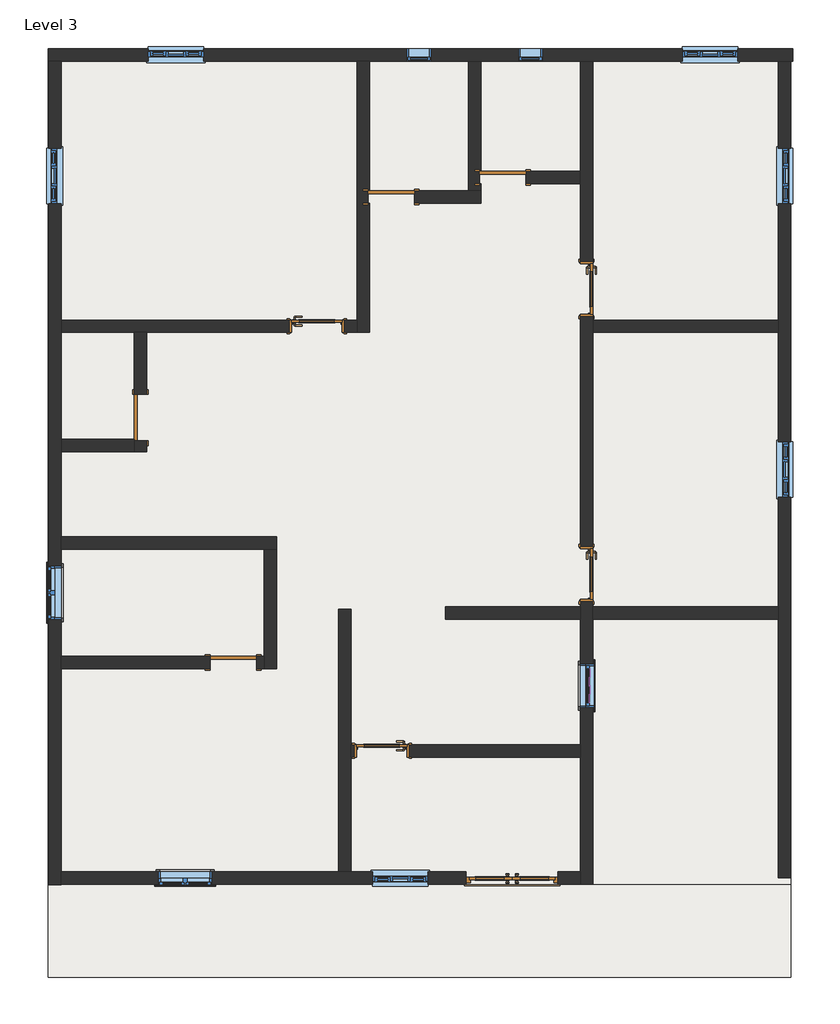
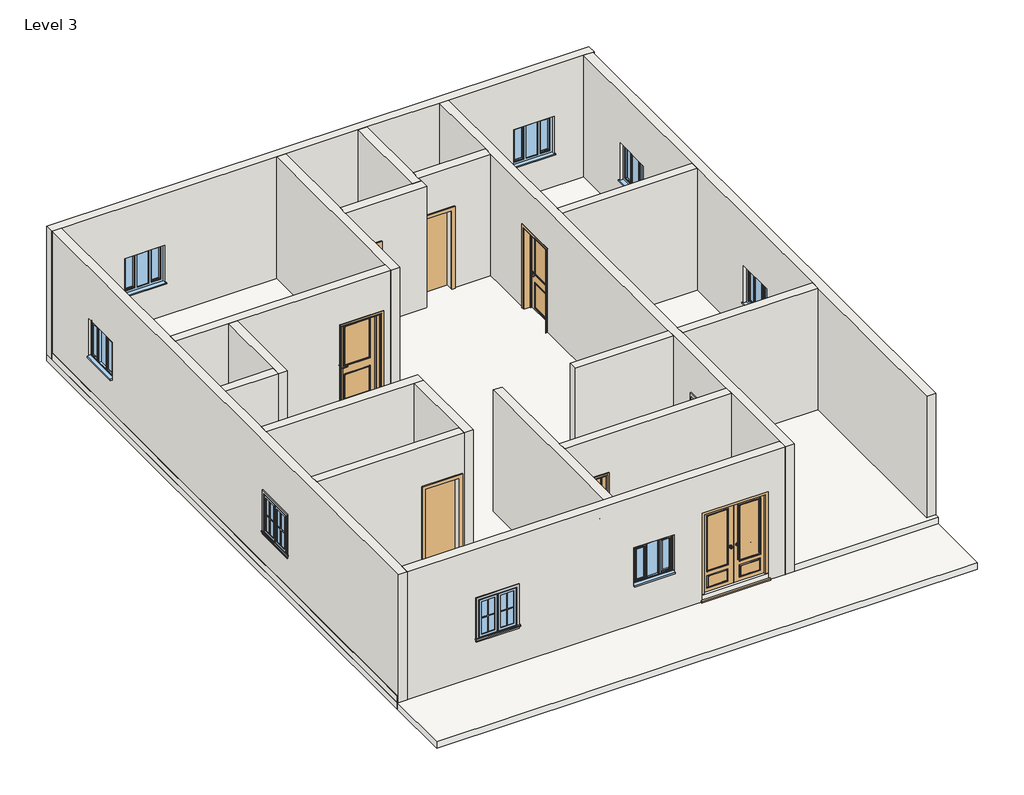
# One storey, incomplete: 19 walls, 12 proxies, 11 windows, 9 doors, 2 slabs, 1 roof.
"""IFC4 building model written with IfcOpenShell, lengths in millimetres."""

from ifc_helpers import new_model, si_unit, frame, origin, place, context, project, spatial, polyline, outline, extrude, faceted_brep, transform, mapped, element, save
from components import muntin_pattern_2x2_muntin_pattern_2x2_b3fe6957, muntin_pattern_2x2_muntin_pattern_2x2_3e0ecaf2, muntin_pattern_2x2_muntin_pattern_2x2_5f474966, trim_window_exterior_flat_with_sill_41619996, trim_window_exterior_flat_with_sill_68241f6a, trim_window_interior_flat_picture_frame_51c85655, trim_window_interior_flat_picture_frame_d3d93820, doors_extdbl_w_glazing_bars_2_1510x2110mm_e5cd3545, doors_extdbl_w_glazing_bars_2_1510x2110mm_b3535315, doors_intsgl_w_transome_910x2110mm_1071bad6, doors_intsgl_w_transome_910x2110mm_0d7ac49b, door_fadea3f2, door_53b1b562, window_085f26e1, window_c29befe5, window_4d695ea9, windows_tpl_plain_910x910mm_84e79c20

model = new_model("IFC4")

# Units and contexts
model_context = context("Model", 3, world=origin())
ifc_project = project(units=[si_unit("LENGTHUNIT", "METRE", prefix="MILLI")], contexts=[model_context])

# Site, building, storey
site = spatial("IfcSite", under=ifc_project)
building = spatial("IfcBuilding", under=site)
storey = spatial("IfcBuildingStorey", under=building, Name="Level 3", Elevation=6096.0)

# Proxies
placement = place(None, origin())
muntin_pattern_2x2_muntin_pattern_2x2_shape = muntin_pattern_2x2_muntin_pattern_2x2_b3fe6957(model_context)
element("IfcBuildingElementProxy", 1, Name="Muntin Pattern_2x2 : Muntin Pattern_2x2", ObjectType="Muntin Pattern_2x2 : Muntin Pattern_2x2", at=placement, inside=storey, context=model_context, shape_type="MappedRepresentation", body=[
    mapped(muntin_pattern_2x2_muntin_pattern_2x2_shape, transform((-4444.3565281, -6259.9254533, 7080.25), x_axis=(-1.0, 0.0, 0.0), y_axis=(0.0, -1.0, 0.0), z_axis=(0.0, 0.0, 1.0))),
])
element("IfcBuildingElementProxy", 2, Name="Muntin Pattern_2x2 : Muntin Pattern_2x2", ObjectType="Muntin Pattern_2x2 : Muntin Pattern_2x2", at=placement, inside=storey, context=model_context, shape_type="MappedRepresentation", body=[
    mapped(muntin_pattern_2x2_muntin_pattern_2x2_shape, transform((-6884.3440281, -1708.5629533, 7080.25), x_axis=(0.0, 1.0, 0.0), y_axis=(-1.0, 0.0, 0.0), z_axis=(0.0, 0.0, 1.0))),
])
muntin_pattern_2x2_muntin_pattern_2x2_2_shape = muntin_pattern_2x2_muntin_pattern_2x2_3e0ecaf2(model_context)
element("IfcBuildingElementProxy", 3, Name="Muntin Pattern_2x2 : Muntin Pattern_2x2", ObjectType="Muntin Pattern_2x2 : Muntin Pattern_2x2", at=placement, inside=storey, context=model_context, shape_type="MappedRepresentation", body=[
    mapped(muntin_pattern_2x2_muntin_pattern_2x2_2_shape, transform((-4872.9815281, -6259.9254533, 7080.25), x_axis=(1.0, 0.0, 0.0), y_axis=(0.0, 1.0, 0.0), z_axis=(0.0, 0.0, 1.0))),
])
element("IfcBuildingElementProxy", 4, Name="Muntin Pattern_2x2 : Muntin Pattern_2x2", ObjectType="Muntin Pattern_2x2 : Muntin Pattern_2x2", at=placement, inside=storey, context=model_context, shape_type="MappedRepresentation", body=[
    mapped(muntin_pattern_2x2_muntin_pattern_2x2_2_shape, transform((-6884.3440281, -1279.9379533, 7080.25), x_axis=(0.0, -1.0, 0.0), y_axis=(1.0, 0.0, 0.0), z_axis=(0.0, 0.0, 1.0))),
])
muntin_pattern_2x2_muntin_pattern_2x2_3_shape = muntin_pattern_2x2_muntin_pattern_2x2_5f474966(model_context)
element("IfcBuildingElementProxy", 5, Name="Muntin Pattern_2x2 : Muntin Pattern_2x2", ObjectType="Muntin Pattern_2x2 : Muntin Pattern_2x2", at=placement, inside=storey, context=model_context, shape_type="MappedRepresentation", body=[
    mapped(muntin_pattern_2x2_muntin_pattern_2x2_3_shape, transform((1989.809459, -3018.2504533, 7616.825), x_axis=(0.0, -1.0, 0.0), y_axis=(1.0, 0.0, 0.0), z_axis=(0.0, 0.0, 1.0))),
])
element("IfcBuildingElementProxy", 6, Name="Muntin Pattern_2x2 : Muntin Pattern_2x2", ObjectType="Muntin Pattern_2x2 : Muntin Pattern_2x2", at=placement, inside=storey, context=model_context, shape_type="MappedRepresentation", body=[
    mapped(muntin_pattern_2x2_muntin_pattern_2x2_3_shape, transform((1945.359459, -3018.2504533, 7086.6), x_axis=(0.0, -1.0, 0.0), y_axis=(1.0, 0.0, 0.0), z_axis=(0.0, 0.0, 1.0))),
])
trim_window_exterior_flat_with_sill_shape = trim_window_exterior_flat_with_sill_41619996(model_context)
element("IfcBuildingElementProxy", 7, Name="Trim-Window-Exterior-Flat : with Sill", ObjectType="Trim-Window-Exterior-Flat : with Sill", at=placement, inside=storey, context=model_context, shape_type="MappedRepresentation", body=[
    mapped(trim_window_exterior_flat_with_sill_shape, transform((-4658.6690281, -6269.4504533, 7924.8), x_axis=(1.0, 0.0, 0.0), y_axis=(0.0, 0.0, 1.0), z_axis=(0.0, -1.0, 0.0))),
])
element("IfcBuildingElementProxy", 8, Name="Trim-Window-Exterior-Flat : with Sill", ObjectType="Trim-Window-Exterior-Flat : with Sill", at=placement, inside=storey, context=model_context, shape_type="MappedRepresentation", body=[
    mapped(trim_window_exterior_flat_with_sill_shape, transform((-6893.8690281, -1494.2504533, 7924.8), x_axis=(0.0, -1.0, 0.0), y_axis=(0.0, 0.0, 1.0), z_axis=(-1.0, 0.0, 0.0))),
])
trim_window_exterior_flat_with_sill_2_shape = trim_window_exterior_flat_with_sill_68241f6a(model_context)
element("IfcBuildingElementProxy", 9, Name="Trim-Window-Exterior-Flat : with Sill", ObjectType="Trim-Window-Exterior-Flat : with Sill", at=placement, inside=storey, context=model_context, shape_type="MappedRepresentation", body=[
    mapped(trim_window_exterior_flat_with_sill_2_shape, transform((2024.734459, -3018.2504533, 8178.8), x_axis=(0.0, 1.0, 0.0), y_axis=(0.0, 0.0, 1.0), z_axis=(1.0, 0.0, 0.0))),
])
trim_window_interior_flat_picture_frame_shape = trim_window_interior_flat_picture_frame_51c85655(model_context)
element("IfcBuildingElementProxy", 10, Name="Trim-Window-Interior-Flat : Picture Frame", ObjectType="Trim-Window-Interior-Flat : Picture Frame", at=placement, inside=storey, context=model_context, shape_type="MappedRepresentation", body=[
    mapped(trim_window_interior_flat_picture_frame_shape, transform((-4658.6690281, -6066.2504533, 7924.8), x_axis=(-1.0, 0.0, 0.0), y_axis=(0.0, 0.0, 1.0), z_axis=(0.0, 1.0, 0.0))),
])
element("IfcBuildingElementProxy", 11, Name="Trim-Window-Interior-Flat : Picture Frame", ObjectType="Trim-Window-Interior-Flat : Picture Frame", at=placement, inside=storey, context=model_context, shape_type="MappedRepresentation", body=[
    mapped(trim_window_interior_flat_picture_frame_shape, transform((-6690.6690281, -1494.2504533, 7924.8), x_axis=(0.0, 1.0, 0.0), y_axis=(0.0, 0.0, 1.0), z_axis=(1.0, 0.0, 0.0))),
])
trim_window_interior_flat_picture_frame_2_shape = trim_window_interior_flat_picture_frame_d3d93820(model_context)
element("IfcBuildingElementProxy", 12, Name="Trim-Window-Interior-Flat : Picture Frame", ObjectType="Trim-Window-Interior-Flat : Picture Frame", at=placement, inside=storey, context=model_context, shape_type="MappedRepresentation", body=[
    mapped(trim_window_interior_flat_picture_frame_2_shape, transform((1821.534459, -3018.2504533, 8178.8), x_axis=(0.0, -1.0, 0.0), y_axis=(0.0, 0.0, 1.0), z_axis=(-1.0, 0.0, 0.0))),
])

# Doors
doors_extdbl_w_glazing_bars_2_1510x2110mm_shape = doors_extdbl_w_glazing_bars_2_1510x2110mm_e5cd3545(model_context)
doors_extdbl_w_glazing_bars_2_1510x2110mm_2_shape = doors_extdbl_w_glazing_bars_2_1510x2110mm_b3535315(model_context)
element("IfcDoor", 13, ObjectType="Doors_ExtDbl_w-Glazing_Bars_2 : 1510x2110mm", at=placement, inside=storey, context=model_context, shape_type="MappedRepresentation", body=[
    mapped(doors_extdbl_w_glazing_bars_2_1510x2110mm_shape, transform((703.934459, -6167.8504533, 6096.0), x_axis=(-1.0, 0.0, 0.0), y_axis=(0.0, -1.0, 0.0), z_axis=(0.0, 0.0, 1.0))),
    mapped(doors_extdbl_w_glazing_bars_2_1510x2110mm_2_shape, transform((703.934459, -6167.8504533, 6096.0), x_axis=(-1.0, 0.0, 0.0), y_axis=(0.0, -1.0, 0.0), z_axis=(0.0, 0.0, 1.0))),
])
doors_intsgl_w_transome_910x2110mm_shape = doors_intsgl_w_transome_910x2110mm_1071bad6(model_context)
element("IfcDoor", 14, ObjectType="Doors_IntSgl_w-Transome : 910x2110mm", at=placement, inside=storey, context=model_context, shape_type="MappedRepresentation", body=[
    mapped(doors_intsgl_w_transome_910x2110mm_shape, transform((-1432.8690281, -4085.0504533, 6096.0), x_axis=(-1.0, 0.0, 0.0), y_axis=(0.0, -1.0, 0.0), z_axis=(0.0, 0.0, 1.0))),
])
doors_intsgl_w_transome_910x2110mm_2_shape = doors_intsgl_w_transome_910x2110mm_0d7ac49b(model_context)
element("IfcDoor", 15, ObjectType="Doors_IntSgl_w-Transome : 910x2110mm", at=placement, inside=storey, context=model_context, shape_type="MappedRepresentation", body=[
    mapped(doors_intsgl_w_transome_910x2110mm_2_shape, transform((-2499.6690281, 2874.5495467, 6096.0), x_axis=(1.0, 0.0, 0.0), y_axis=(0.0, 1.0, 0.0), z_axis=(0.0, 0.0, 1.0))),
])
element("IfcDoor", 16, ObjectType="Doors_IntSgl_w-Transome : 910x2110mm", at=placement, inside=storey, context=model_context, shape_type="MappedRepresentation", body=[
    mapped(doors_intsgl_w_transome_910x2110mm_2_shape, transform((1923.134459, 3484.1495467, 6096.0), x_axis=(0.0, -1.0, 0.0), y_axis=(1.0, 0.0, 0.0), z_axis=(0.0, 0.0, 1.0))),
])
element("IfcDoor", 17, ObjectType="Doors_IntSgl_w-Transome : 910x2110mm", at=placement, inside=storey, context=model_context, shape_type="MappedRepresentation", body=[
    mapped(doors_intsgl_w_transome_910x2110mm_2_shape, transform((1923.134459, -1189.4504533, 6096.0), x_axis=(0.0, -1.0, 0.0), y_axis=(1.0, 0.0, 0.0), z_axis=(0.0, 0.0, 1.0))),
])
door_shape = door_fadea3f2(model_context)
element("IfcDoor", 18, ObjectType="Single-Flush : 30\" x 80\"", at=placement, inside=storey, context=model_context, shape_type="MappedRepresentation", body=[
    mapped(door_shape, transform((-3871.2690281, -2637.2504533, 6096.0), x_axis=(1.0, 0.0, 0.0), y_axis=(0.0, 1.0, 0.0), z_axis=(0.0, 0.0, 1.0))),
])
door_2_shape = door_53b1b562(model_context)
element("IfcDoor", 19, ObjectType="Single-Flush : 30\" x 80\"", at=placement, inside=storey, context=model_context, shape_type="MappedRepresentation", body=[
    mapped(door_2_shape, transform((-5395.2690281, 1375.9495467, 6096.0), x_axis=(0.0, -1.0, 0.0), y_axis=(1.0, 0.0, 0.0), z_axis=(0.0, 0.0, 1.0))),
])
element("IfcDoor", 20, ObjectType="Single-Flush : 30\" x 80\"", at=placement, inside=storey, context=model_context, shape_type="MappedRepresentation", body=[
    mapped(door_2_shape, transform((-1280.4690281, 4995.4495467, 6096.0), x_axis=(-1.0, 0.0, 0.0), y_axis=(0.0, -1.0, 0.0), z_axis=(0.0, 0.0, 1.0))),
])
element("IfcDoor", 21, ObjectType="Single-Flush : 30\" x 80\"", at=placement, inside=storey, context=model_context, shape_type="MappedRepresentation", body=[
    mapped(door_2_shape, transform((548.3309719, 5312.9495467, 6096.0), x_axis=(-1.0, 0.0, 0.0), y_axis=(0.0, -1.0, 0.0), z_axis=(0.0, 0.0, 1.0))),
])

# Roof
element("IfcRoof", 22, ObjectType="Generic - 12\"", at=placement, inside=storey, context=model_context, shape_type="SweptSolid", body=[
    extrude(outline(polyline([(-6906.5690281, 7421.1495467), (5272.7309719, 7421.1495467), (5272.7309719, -6269.4504533), (-6906.5690281, -6269.4504533), (-6906.5690281, 7421.1495467)])), frame((0.0, 0.0, 6096.0), z_axis=(0.0, 0.0, 1.0), x_axis=(1.0, 0.0, 0.0)), (0.0, 0.0, 1.0), 152.4),
])

# Slabs
element("IfcSlab", 23, ObjectType="Generic - 12\"", at=placement, inside=storey, context=model_context, shape_type="SweptSolid", body=[
    extrude(outline(polyline([(5272.7309719, 7421.1495467), (5272.7309719, -6269.4504533), (-6906.5690281, -6269.4504533), (-6906.5690281, 7421.1495467), (5272.7309719, 7421.1495467)])), frame((0.0, 0.0, 5943.6), z_axis=(0.0, 0.0, 1.0), x_axis=(1.0, 0.0, 0.0)), (0.0, 0.0, 1.0), 152.4),
])
element("IfcSlab", 24, ObjectType="Generic - 12\"", at=placement, inside=storey, context=model_context, shape_type="SweptSolid", body=[
    extrude(outline(polyline([(5272.7309719, -6269.4504533), (5272.7309719, -7799.0240652), (-6906.5690281, -7799.0240652), (-6906.5690281, -6269.4504533), (5272.7309719, -6269.4504533)])), frame((0.0, 0.0, 5943.6), z_axis=(0.0, 0.0, 1.0), x_axis=(1.0, 0.0, 0.0)), (0.0, 0.0, 1.0), 152.4),
])

# Walls
element("IfcWall", 25, ObjectType="4.5\" p", at=placement, inside=storey, context=model_context, shape_type="Brep", body=[
    faceted_brep([(-1839.2690281, 7217.9495467, 6096.0), (-1839.2690281, 2976.1495467, 6096.0), (-1839.2690281, 2772.9495467, 6096.0), (-1839.2690281, 2772.9495467, 9144.0), (-1839.2690281, 2976.1495467, 9144.0), (-1839.2690281, 7217.9495467, 9144.0), (-1636.0690281, 7217.9495467, 9144.0), (-1636.0690281, 5097.0495467, 9144.0), (-1636.0690281, 4893.8495467, 9144.0), (-1636.0690281, 2772.9495467, 9144.0), (-1636.0690281, 2772.9495467, 6096.0), (-1636.0690281, 4893.8495467, 6096.0), (-1636.0690281, 4893.8495467, 8128.0), (-1636.0690281, 5097.0495467, 8128.0), (-1636.0690281, 5097.0495467, 6096.0), (-1636.0690281, 7217.9495467, 6096.0), (-1661.4690281, 5097.0495467, 6096.0), (-1661.4690281, 4893.8495467, 6096.0), (-1661.4690281, 5097.0495467, 8128.0), (-1661.4690281, 4893.8495467, 8128.0)], [[[0, 1, 2, 3, 4, 5]], [[6, 7, 8, 9, 10, 11, 12, 13, 14, 15]], [[2, 1, 0, 15, 14, 16, 17, 11, 10]], [[5, 4, 3, 9, 8, 7, 6]], [[0, 5, 6, 15]], [[3, 2, 10, 9]], [[18, 16, 14, 13]], [[17, 19, 12, 11]], [[19, 18, 13, 12]], [[16, 18, 19, 17]]]),
])
element("IfcWall", 26, ObjectType="4.5\" p", at=placement, inside=storey, context=model_context, shape_type="Brep", body=[
    faceted_brep([(-1839.2690281, 2772.9495467, 9144.0), (-5293.6690281, 2772.9495467, 9144.0), (-5496.8690281, 2772.9495467, 9144.0), (-6690.6690281, 2772.9495467, 9144.0), (-6690.6690281, 2772.9495467, 6096.0), (-5496.8690281, 2772.9495467, 6096.0), (-5293.6690281, 2772.9495467, 6096.0), (-2954.6690281, 2772.9495467, 6096.0), (-2954.6690281, 2772.9495467, 8206.0), (-2044.6690281, 2772.9495467, 8206.0), (-2044.6690281, 2772.9495467, 6096.0), (-1839.2690281, 2772.9495467, 6096.0), (-6690.6690281, 2976.1495467, 9144.0), (-1839.2690281, 2976.1495467, 9144.0), (-1839.2690281, 2976.1495467, 6096.0), (-2044.6690281, 2976.1495467, 6096.0), (-2044.6690281, 2976.1495467, 8206.0), (-2954.6690281, 2976.1495467, 8206.0), (-2954.6690281, 2976.1495467, 6096.0), (-6690.6690281, 2976.1495467, 6096.0)], [[[0, 1, 2, 3, 4, 5, 6, 7, 8, 9, 10, 11]], [[12, 13, 14, 15, 16, 17, 18, 19]], [[4, 19, 18, 7, 6, 5]], [[14, 11, 10, 15]], [[3, 2, 1, 0, 13, 12]], [[0, 11, 14, 13]], [[4, 3, 12, 19]], [[9, 16, 15, 10]], [[16, 9, 8, 17]], [[17, 8, 7, 18]]]),
])
element("IfcWall", 27, ObjectType="4.5\" p", at=placement, inside=storey, context=model_context, shape_type="Brep", body=[
    faceted_brep([(-5496.8690281, 994.9495467, 8128.0), (-5496.8690281, 994.9495467, 6096.0), (-5496.8690281, 817.1495467, 6096.0), (-5496.8690281, 817.1495467, 9144.0), (-5496.8690281, 1020.3495467, 9144.0), (-5496.8690281, 2772.9495467, 9144.0), (-5496.8690281, 2772.9495467, 6096.0), (-5496.8690281, 1756.9495467, 6096.0), (-5496.8690281, 1756.9495467, 8128.0), (-5293.6690281, 817.1495467, 6096.0), (-5293.6690281, 994.9495467, 6096.0), (-5293.6690281, 994.9495467, 8128.0), (-5293.6690281, 1756.9495467, 8128.0), (-5293.6690281, 1756.9495467, 6096.0), (-5293.6690281, 2772.9495467, 6096.0), (-5293.6690281, 2772.9495467, 9144.0), (-5293.6690281, 817.1495467, 9144.0)], [[[0, 1, 2, 3, 4, 5, 6, 7, 8]], [[9, 10, 11, 12, 13, 14, 15, 16]], [[7, 6, 14, 13]], [[2, 1, 10, 9]], [[5, 4, 3, 16, 15]], [[6, 5, 15, 14]], [[3, 2, 9, 16]], [[11, 10, 1, 0]], [[12, 11, 0, 8]], [[13, 12, 8, 7]]]),
])
element("IfcWall", 28, ObjectType="4.5\" p", at=placement, inside=storey, context=model_context, shape_type="SweptSolid", body=[
    extrude(outline(polyline([(-5496.8690281, 817.1495467), (-6690.6690281, 817.1495467), (-6690.6690281, 1020.3495467), (-5496.8690281, 1020.3495467), (-5496.8690281, 817.1495467)])), frame((0.0, 0.0, 6096.0), z_axis=(0.0, 0.0, 1.0), x_axis=(1.0, 0.0, 0.0)), (0.0, 0.0, 1.0), 3048.0),
])
element("IfcWall", 29, ObjectType="4.5\" p", at=placement, inside=storey, context=model_context, shape_type="Brep", body=[
    faceted_brep([(-6690.6690281, -783.0504533, 6096.0), (-3363.2690281, -783.0504533, 6096.0), (-3160.0690281, -783.0504533, 6096.0), (-3160.0690281, -783.0504533, 9144.0), (-3363.2690281, -783.0504533, 9144.0), (-6690.6690281, -783.0504533, 9144.0), (-6690.6690281, -579.8504533, 6096.0), (-6690.6690281, -579.8504533, 9144.0), (-3160.0690281, -579.8504533, 9144.0), (-3160.0690281, -579.8504533, 6096.0)], [[[0, 1, 2, 3, 4, 5]], [[6, 7, 8, 9]], [[2, 1, 0, 6, 9]], [[5, 4, 3, 8, 7]], [[0, 5, 7, 6]], [[3, 2, 9, 8]]]),
])
element("IfcWall", 30, ObjectType="4.5\" p", at=placement, inside=storey, context=model_context, shape_type="Brep", body=[
    faceted_brep([(-3363.2690281, -783.0504533, 6096.0), (-3363.2690281, -2535.6504533, 6096.0), (-3363.2690281, -2738.8504533, 6096.0), (-3363.2690281, -2738.8504533, 9144.0), (-3363.2690281, -2535.6504533, 9144.0), (-3363.2690281, -783.0504533, 9144.0), (-3160.0690281, -783.0504533, 6096.0), (-3160.0690281, -783.0504533, 9144.0), (-3160.0690281, -2738.8504533, 9144.0), (-3160.0690281, -2738.8504533, 6096.0)], [[[0, 1, 2, 3, 4, 5]], [[6, 7, 8, 9]], [[2, 1, 0, 6, 9]], [[5, 4, 3, 8, 7]], [[0, 5, 7, 6]], [[3, 2, 9, 8]]]),
])
element("IfcWall", 31, ObjectType="4.5\" p", at=placement, inside=storey, context=model_context, shape_type="SweptSolid", body=[
    extrude(outline(polyline([(8128.0, -3490.2690281), (6096.0, -3490.2690281), (6096.0, -3363.2690281), (9144.0, -3363.2690281), (9144.0, -6690.6690281), (6096.0, -6690.6690281), (6096.0, -4252.2690281), (8128.0, -4252.2690281), (8128.0, -3490.2690281)])), frame((0.0, -2738.8504533, 0.0), z_axis=(0.0, 1.0, 0.0), x_axis=(0.0, 0.0, 1.0)), (0.0, 0.0, 1.0), 203.2),
])
element("IfcWall", 32, ObjectType="4.5\" p", at=placement, inside=storey, context=model_context, shape_type="Brep", body=[
    faceted_brep([(192.7309719, 4893.8495467, 9144.0), (-1636.0690281, 4893.8495467, 9144.0), (-1636.0690281, 4893.8495467, 8128.0), (-899.4690281, 4893.8495467, 8128.0), (-899.4690281, 4893.8495467, 6096.0), (192.7309719, 4893.8495467, 6096.0), (-1636.0690281, 5097.0495467, 9144.0), (-10.4690281, 5097.0495467, 9144.0), (192.7309719, 5097.0495467, 9144.0), (192.7309719, 5097.0495467, 6096.0), (-10.4690281, 5097.0495467, 6096.0), (-899.4690281, 5097.0495467, 6096.0), (-899.4690281, 5097.0495467, 8128.0), (-1636.0690281, 5097.0495467, 8128.0)], [[[0, 1, 2, 3, 4, 5]], [[6, 7, 8, 9, 10, 11, 12, 13]], [[9, 5, 4, 11, 10]], [[1, 0, 8, 7, 6]], [[1, 6, 13, 2]], [[0, 5, 9, 8]], [[12, 3, 2, 13]], [[3, 12, 11, 4]]]),
])
element("IfcWall", 33, ObjectType="4.5\" p", at=placement, inside=storey, context=model_context, shape_type="Brep", body=[
    faceted_brep([(-10.4690281, 7217.9495467, 6096.0), (-10.4690281, 5097.0495467, 6096.0), (-10.4690281, 5097.0495467, 9144.0), (-10.4690281, 7217.9495467, 9144.0), (192.7309719, 7217.9495467, 9144.0), (192.7309719, 5414.5495467, 9144.0), (192.7309719, 5211.3495467, 9144.0), (192.7309719, 5097.0495467, 9144.0), (192.7309719, 5097.0495467, 6096.0), (192.7309719, 5211.3495467, 6096.0), (192.7309719, 5211.3495467, 8128.0), (192.7309719, 5414.5495467, 8128.0), (192.7309719, 5414.5495467, 6096.0), (192.7309719, 7217.9495467, 6096.0), (167.3309719, 5414.5495467, 6096.0), (167.3309719, 5211.3495467, 6096.0), (167.3309719, 5414.5495467, 8128.0), (167.3309719, 5211.3495467, 8128.0)], [[[0, 1, 2, 3]], [[4, 5, 6, 7, 8, 9, 10, 11, 12, 13]], [[1, 0, 13, 12, 14, 15, 9, 8]], [[3, 2, 7, 6, 5, 4]], [[2, 1, 8, 7]], [[0, 3, 4, 13]], [[16, 14, 12, 11]], [[15, 17, 10, 9]], [[17, 16, 11, 10]], [[14, 16, 17, 15]]]),
])
element("IfcWall", 34, ObjectType="4.5\" p", at=placement, inside=storey, context=model_context, shape_type="Brep", body=[
    faceted_brep([(1821.534459, -6269.4504533, 9144.0), (1821.534459, -6066.2504533, 9144.0), (1821.534459, -4186.6504533, 9144.0), (1821.534459, -3983.4504533, 9144.0), (1821.534459, -1926.0504533, 9144.0), (1821.534459, -1722.8504533, 9144.0), (1821.534459, 5211.3495467, 9144.0), (1821.534459, 5414.5495467, 9144.0), (1821.534459, 7217.9495467, 9144.0), (1821.534459, 7217.9495467, 6096.0), (1821.534459, 5414.5495467, 6096.0), (1821.534459, 5211.3495467, 6096.0), (1821.534459, 3939.1495467, 6096.0), (1821.534459, 3939.1495467, 8206.0), (1821.534459, 3029.1495467, 8206.0), (1821.534459, 3029.1495467, 6096.0), (1821.534459, -734.4504533, 6096.0), (1821.534459, -734.4504533, 8206.0), (1821.534459, -1644.4504533, 8206.0), (1821.534459, -1644.4504533, 6096.0), (1821.534459, -1722.8504533, 6096.0), (1821.534459, -1926.0504533, 6096.0), (1821.534459, -3983.4504533, 6096.0), (1821.534459, -4186.6504533, 6096.0), (1821.534459, -6066.2504533, 6096.0), (1821.534459, -6269.4504533, 6096.0), (1821.534459, -2662.6504533, 8178.8), (1821.534459, -3373.8504533, 8178.8), (1821.534459, -3373.8504533, 7010.4), (1821.534459, -2662.6504533, 7010.4), (2024.734459, 7217.9495467, 9144.0), (2024.734459, 2976.1495467, 9144.0), (2024.734459, 2772.9495467, 9144.0), (2024.734459, -1722.8504533, 9144.0), (2024.734459, -1926.0504533, 9144.0), (2024.734459, -6269.4504533, 9144.0), (2024.734459, -6269.4504533, 6096.0), (2024.734459, -1926.0504533, 6096.0), (2024.734459, -1722.8504533, 6096.0), (2024.734459, -1644.4504533, 6096.0), (2024.734459, -1644.4504533, 8206.0), (2024.734459, -734.4504533, 8206.0), (2024.734459, -734.4504533, 6096.0), (2024.734459, 2772.9495467, 6096.0), (2024.734459, 2976.1495467, 6096.0), (2024.734459, 3029.1495467, 6096.0), (2024.734459, 3029.1495467, 8206.0), (2024.734459, 3939.1495467, 8206.0), (2024.734459, 3939.1495467, 6096.0), (2024.734459, 7217.9495467, 6096.0), (2024.734459, -2662.6504533, 8178.8), (2024.734459, -2662.6504533, 7010.4), (2024.734459, -3373.8504533, 7010.4), (2024.734459, -3373.8504533, 8178.8)], [[[0, 1, 2, 3, 4, 5, 6, 7, 8, 9, 10, 11, 12, 13, 14, 15, 16, 17, 18, 19, 20, 21, 22, 23, 24, 25], [26, 27, 28, 29]], [[30, 31, 32, 33, 34, 35, 36, 37, 38, 39, 40, 41, 42, 43, 44, 45, 46, 47, 48, 49], [50, 51, 52, 53]], [[9, 49, 48, 12, 11, 10]], [[15, 45, 44, 43, 42, 16]], [[36, 25, 24, 23, 22, 21, 20, 19, 39, 38, 37]], [[8, 7, 6, 5, 4, 3, 2, 1, 0, 35, 34, 33, 32, 31, 30]], [[9, 8, 30, 49]], [[14, 46, 45, 15]], [[46, 14, 13, 47]], [[47, 13, 12, 48]], [[18, 40, 39, 19]], [[40, 18, 17, 41]], [[41, 17, 16, 42]], [[0, 25, 36, 35]], [[51, 50, 26, 29]], [[52, 51, 29, 28]], [[53, 52, 28, 27]], [[50, 53, 27, 26]]]),
])
element("IfcWall", 35, ObjectType="4.5\" p", at=placement, inside=storey, context=model_context, shape_type="SweptSolid", body=[
    extrude(outline(polyline([(-391.4690281, -1926.0504533), (-391.4690281, -1722.8504533), (1821.534459, -1722.8504533), (1821.534459, -1926.0504533), (-391.4690281, -1926.0504533)])), frame((0.0, 0.0, 6096.0), z_axis=(0.0, 0.0, 1.0), x_axis=(1.0, 0.0, 0.0)), (0.0, 0.0, 1.0), 3048.0),
    extrude(outline(polyline([(5069.5309719, -1722.8504533), (5069.5309719, -1926.0504533), (2024.734459, -1926.0504533), (2024.734459, -1722.8504533), (5069.5309719, -1722.8504533)])), frame((0.0, 0.0, 6096.0), z_axis=(0.0, 0.0, 1.0), x_axis=(1.0, 0.0, 0.0)), (0.0, 0.0, 1.0), 3048.0),
])
element("IfcWall", 36, ObjectType="4.5\" p", at=placement, inside=storey, context=model_context, shape_type="SweptSolid", body=[
    extrude(outline(polyline([(5069.5309719, 2772.9495467), (2024.734459, 2772.9495467), (2024.734459, 2976.1495467), (5069.5309719, 2976.1495467), (5069.5309719, 2772.9495467)])), frame((0.0, 0.0, 6096.0), z_axis=(0.0, 0.0, 1.0), x_axis=(1.0, 0.0, 0.0)), (0.0, 0.0, 1.0), 3048.0),
])
element("IfcWall", 37, ObjectType="4.5\" p", at=placement, inside=storey, context=model_context, shape_type="SweptSolid", body=[
    extrude(outline(polyline([(9144.0, 1821.534459), (9144.0, 192.7309719), (8128.0, 192.7309719), (8128.0, 929.3309719), (6096.0, 929.3309719), (6096.0, 1821.534459), (9144.0, 1821.534459)])), frame((0.0, 5211.3495467, 0.0), z_axis=(0.0, 1.0, 0.0), x_axis=(0.0, 0.0, 1.0)), (0.0, 0.0, 1.0), 203.2),
])
element("IfcWall", 38, ObjectType="4.5\" p", at=placement, inside=storey, context=model_context, shape_type="Brep", body=[
    faceted_brep([(-1940.8690281, -6066.2504533, 6096.0), (-1940.8690281, -4186.6504533, 6096.0), (-1940.8690281, -3983.4504533, 6096.0), (-1940.8690281, -1760.9504533, 6096.0), (-1940.8690281, -1760.9504533, 9144.0), (-1940.8690281, -3983.4504533, 9144.0), (-1940.8690281, -4186.6504533, 9144.0), (-1940.8690281, -6066.2504533, 9144.0), (-2144.0690281, -6066.2504533, 6096.0), (-2144.0690281, -6066.2504533, 9144.0), (-2144.0690281, -1760.9504533, 9144.0), (-2144.0690281, -1760.9504533, 6096.0)], [[[0, 1, 2, 3, 4, 5, 6, 7]], [[8, 9, 10, 11]], [[3, 2, 1, 0, 8, 11]], [[4, 3, 11, 10]], [[7, 6, 5, 4, 10, 9]], [[0, 7, 9, 8]]]),
])
element("IfcWall", 39, ObjectType="4.5\" p", at=placement, inside=storey, context=model_context, shape_type="SweptSolid", body=[
    extrude(outline(polyline([(9144.0, 1821.534459), (9144.0, -1940.8690281), (6096.0, -1940.8690281), (6096.0, -1887.8690281), (8206.0, -1887.8690281), (8206.0, -977.8690281), (6096.0, -977.8690281), (6096.0, 1821.534459), (9144.0, 1821.534459)])), frame((0.0, -4186.6504533, 0.0), z_axis=(0.0, 1.0, 0.0), x_axis=(0.0, 0.0, 1.0)), (0.0, 0.0, 1.0), 203.2),
])
element("IfcWall", 40, ObjectType="9\"", at=placement, inside=storey, context=model_context, shape_type="Brep", body=[
    faceted_brep([(5069.5309719, 7217.9495467, 6096.0), (5069.5309719, 2976.1495467, 6096.0), (5069.5309719, 2772.9495467, 6096.0), (5069.5309719, -1722.8504533, 6096.0), (5069.5309719, -1926.0504533, 6096.0), (5069.5309719, -6167.8504533, 6096.0), (5069.5309719, -6167.8504533, 9144.0), (5069.5309719, -1926.0504533, 9144.0), (5069.5309719, -1722.8504533, 9144.0), (5069.5309719, 2772.9495467, 9144.0), (5069.5309719, 2976.1495467, 9144.0), (5069.5309719, 7217.9495467, 9144.0), (5069.5309719, 980.0495467, 7920.4), (5069.5309719, 70.0495467, 7920.4), (5069.5309719, 70.0495467, 7010.4), (5069.5309719, 980.0495467, 7010.4), (5069.5309719, 5793.3495467, 7920.4), (5069.5309719, 4883.3495467, 7920.4), (5069.5309719, 4883.3495467, 7010.4), (5069.5309719, 5793.3495467, 7010.4), (5272.7309719, 7217.9495467, 6096.0), (5272.7309719, 7217.9495467, 9144.0), (5272.7309719, -6167.8504533, 9144.0), (5272.7309719, -6167.8504533, 6096.0), (5272.7309719, 980.0495467, 7920.4), (5272.7309719, 980.0495467, 7010.4), (5272.7309719, 70.0495467, 7010.4), (5272.7309719, 70.0495467, 7920.4), (5272.7309719, 5793.3495467, 7920.4), (5272.7309719, 5793.3495467, 7010.4), (5272.7309719, 4883.3495467, 7010.4), (5272.7309719, 4883.3495467, 7920.4)], [[[0, 1, 2, 3, 4, 5, 6, 7, 8, 9, 10, 11], [12, 13, 14, 15], [16, 17, 18, 19]], [[20, 21, 22, 23], [24, 25, 26, 27], [28, 29, 30, 31]], [[5, 4, 3, 2, 1, 0, 20, 23]], [[6, 5, 23, 22]], [[11, 10, 9, 8, 7, 6, 22, 21]], [[0, 11, 21, 20]], [[25, 24, 12, 15]], [[26, 25, 15, 14]], [[27, 26, 14, 13]], [[24, 27, 13, 12]], [[29, 28, 16, 19]], [[30, 29, 19, 18]], [[31, 30, 18, 17]], [[28, 31, 17, 16]]]),
])
element("IfcWall", 41, ObjectType="9\" wall", at=placement, inside=storey, context=model_context, shape_type="Brep", body=[
    faceted_brep([(-6906.5690281, 7217.9495467, 6096.0), (-6893.8690281, 7217.9495467, 6096.0), (-6690.6690281, 7217.9495467, 6096.0), (-1839.2690281, 7217.9495467, 6096.0), (-1636.0690281, 7217.9495467, 6096.0), (-10.4690281, 7217.9495467, 6096.0), (192.7309719, 7217.9495467, 6096.0), (1821.534459, 7217.9495467, 6096.0), (2024.734459, 7217.9495467, 6096.0), (5069.5309719, 7217.9495467, 6096.0), (5272.7309719, 7217.9495467, 6096.0), (5310.8309719, 7217.9495467, 6096.0), (5310.8309719, 7217.9495467, 9144.0), (5272.7309719, 7217.9495467, 9144.0), (5069.5309719, 7217.9495467, 9144.0), (2024.734459, 7217.9495467, 9144.0), (1821.534459, 7217.9495467, 9144.0), (192.7309719, 7217.9495467, 9144.0), (-10.4690281, 7217.9495467, 9144.0), (-1636.0690281, 7217.9495467, 9144.0), (-1839.2690281, 7217.9495467, 9144.0), (-6690.6690281, 7217.9495467, 9144.0), (-6893.8690281, 7217.9495467, 9144.0), (-6906.5690281, 7217.9495467, 9144.0), (-5266.0690281, 7217.9495467, 7920.4), (-4356.0690281, 7217.9495467, 7920.4), (-4356.0690281, 7217.9495467, 7010.4), (-5266.0690281, 7217.9495467, 7010.4), (3496.9309719, 7217.9495467, 7920.4), (4406.9309719, 7217.9495467, 7920.4), (4406.9309719, 7217.9495467, 7010.4), (3496.9309719, 7217.9495467, 7010.4), (-1026.4690281, 7217.9495467, 7620.0), (-620.0690281, 7217.9495467, 7620.0), (-620.0690281, 7217.9495467, 7010.4), (-1026.4690281, 7217.9495467, 7010.4), (803.9327155, 7217.9495467, 7620.0), (1210.3327155, 7217.9495467, 7620.0), (1210.3327155, 7217.9495467, 7010.4), (803.9327155, 7217.9495467, 7010.4), (-6906.5690281, 7421.1495467, 6096.0), (-6906.5690281, 7421.1495467, 9144.0), (5310.8309719, 7421.1495467, 9144.0), (5310.8309719, 7421.1495467, 6096.0), (-5266.0690281, 7421.1495467, 7920.4), (-5266.0690281, 7421.1495467, 7010.4), (-4356.0690281, 7421.1495467, 7010.4), (-4356.0690281, 7421.1495467, 7920.4), (3496.9309719, 7421.1495467, 7920.4), (3496.9309719, 7421.1495467, 7010.4), (4406.9309719, 7421.1495467, 7010.4), (4406.9309719, 7421.1495467, 7920.4), (-1026.4690281, 7421.1495467, 7620.0), (-1026.4690281, 7421.1495467, 7010.4), (-620.0690281, 7421.1495467, 7010.4), (-620.0690281, 7421.1495467, 7620.0), (803.9327155, 7421.1495467, 7620.0), (803.9327155, 7421.1495467, 7010.4), (1210.3327155, 7421.1495467, 7010.4), (1210.3327155, 7421.1495467, 7620.0)], [[[0, 1, 2, 3, 4, 5, 6, 7, 8, 9, 10, 11, 12, 13, 14, 15, 16, 17, 18, 19, 20, 21, 22, 23], [24, 25, 26, 27], [28, 29, 30, 31], [32, 33, 34, 35], [36, 37, 38, 39]], [[40, 41, 42, 43], [44, 45, 46, 47], [48, 49, 50, 51], [52, 53, 54, 55], [56, 57, 58, 59]], [[11, 10, 9, 8, 7, 6, 5, 4, 3, 2, 1, 0, 40, 43]], [[12, 11, 43, 42]], [[23, 22, 21, 20, 19, 18, 17, 16, 15, 14, 13, 12, 42, 41]], [[0, 23, 41, 40]], [[45, 44, 24, 27]], [[46, 45, 27, 26]], [[47, 46, 26, 25]], [[44, 47, 25, 24]], [[49, 48, 28, 31]], [[50, 49, 31, 30]], [[51, 50, 30, 29]], [[48, 51, 29, 28]], [[53, 52, 32, 35]], [[54, 53, 35, 34]], [[55, 54, 34, 33]], [[52, 55, 33, 32]], [[57, 56, 36, 39]], [[58, 57, 39, 38]], [[59, 58, 38, 37]], [[56, 59, 37, 36]]]),
])
element("IfcWall", 42, ObjectType="9\" wall", at=placement, inside=storey, context=model_context, shape_type="Brep", body=[
    faceted_brep([(-6893.8690281, 7217.9495467, 6096.0), (-6893.8690281, -6282.1504533, 6096.0), (-6893.8690281, -6282.1504533, 9144.0), (-6893.8690281, 7217.9495467, 9144.0), (-6893.8690281, -1062.4504533, 7924.8), (-6893.8690281, -1926.0504533, 7924.8), (-6893.8690281, -1926.0504533, 7010.4), (-6893.8690281, -1062.4504533, 7010.4), (-6893.8690281, 4883.3495467, 7920.4), (-6893.8690281, 4883.3495467, 7010.4), (-6893.8690281, 5793.3495467, 7010.4), (-6893.8690281, 5793.3495467, 7920.4), (-6690.6690281, 7217.9495467, 6096.0), (-6690.6690281, 7217.9495467, 9144.0), (-6690.6690281, 2976.1495467, 9144.0), (-6690.6690281, 2772.9495467, 9144.0), (-6690.6690281, 1020.3495467, 9144.0), (-6690.6690281, 817.1495467, 9144.0), (-6690.6690281, -579.8504533, 9144.0), (-6690.6690281, -783.0504533, 9144.0), (-6690.6690281, -2535.6504533, 9144.0), (-6690.6690281, -2738.8504533, 9144.0), (-6690.6690281, -6066.2504533, 9144.0), (-6690.6690281, -6269.4504533, 9144.0), (-6690.6690281, -6282.1504533, 9144.0), (-6690.6690281, -6282.1504533, 6096.0), (-6690.6690281, -6269.4504533, 6096.0), (-6690.6690281, -6066.2504533, 6096.0), (-6690.6690281, -2738.8504533, 6096.0), (-6690.6690281, -2535.6504533, 6096.0), (-6690.6690281, -783.0504533, 6096.0), (-6690.6690281, -579.8504533, 6096.0), (-6690.6690281, 817.1495467, 6096.0), (-6690.6690281, 1020.3495467, 6096.0), (-6690.6690281, 2772.9495467, 6096.0), (-6690.6690281, 2976.1495467, 6096.0), (-6690.6690281, -1062.4504533, 7924.8), (-6690.6690281, -1062.4504533, 7010.4), (-6690.6690281, -1926.0504533, 7010.4), (-6690.6690281, -1926.0504533, 7924.8), (-6690.6690281, 4883.3495467, 7920.4), (-6690.6690281, 5793.3495467, 7920.4), (-6690.6690281, 5793.3495467, 7010.4), (-6690.6690281, 4883.3495467, 7010.4)], [[[0, 1, 2, 3], [4, 5, 6, 7], [8, 9, 10, 11]], [[12, 13, 14, 15, 16, 17, 18, 19, 20, 21, 22, 23, 24, 25, 26, 27, 28, 29, 30, 31, 32, 33, 34, 35], [36, 37, 38, 39], [40, 41, 42, 43]], [[1, 0, 12, 35, 34, 33, 32, 31, 30, 29, 28, 27, 26, 25]], [[2, 1, 25, 24]], [[3, 2, 24, 23, 22, 21, 20, 19, 18, 17, 16, 15, 14, 13]], [[0, 3, 13, 12]], [[37, 36, 4, 7]], [[38, 37, 7, 6]], [[39, 38, 6, 5]], [[36, 39, 5, 4]], [[9, 8, 40, 43]], [[10, 9, 43, 42]], [[11, 10, 42, 41]], [[8, 11, 41, 40]]]),
])
element("IfcWall", 43, ObjectType="9\" wall", at=placement, inside=storey, context=model_context, shape_type="Brep", body=[
    faceted_brep([(1821.534459, -6269.4504533, 9144.0), (-6690.6690281, -6269.4504533, 9144.0), (-6690.6690281, -6269.4504533, 6096.0), (-51.065541, -6269.4504533, 6096.0), (-51.065541, -6269.4504533, 8206.0), (1458.934459, -6269.4504533, 8206.0), (1458.934459, -6269.4504533, 6096.0), (1821.534459, -6269.4504533, 6096.0), (-5090.4690281, -6269.4504533, 7924.8), (-4226.8690281, -6269.4504533, 7924.8), (-4226.8690281, -6269.4504533, 7010.4), (-5090.4690281, -6269.4504533, 7010.4), (-673.0690281, -6269.4504533, 7920.4), (-673.0690281, -6269.4504533, 7010.4), (-1583.0690281, -6269.4504533, 7010.4), (-1583.0690281, -6269.4504533, 7920.4), (-6690.6690281, -6066.2504533, 9144.0), (-2144.0690281, -6066.2504533, 9144.0), (-1940.8690281, -6066.2504533, 9144.0), (1821.534459, -6066.2504533, 9144.0), (1821.534459, -6066.2504533, 6096.0), (1458.934459, -6066.2504533, 6096.0), (1458.934459, -6066.2504533, 8206.0), (-51.065541, -6066.2504533, 8206.0), (-51.065541, -6066.2504533, 6096.0), (-1940.8690281, -6066.2504533, 6096.0), (-2144.0690281, -6066.2504533, 6096.0), (-6690.6690281, -6066.2504533, 6096.0), (-5090.4690281, -6066.2504533, 7924.8), (-5090.4690281, -6066.2504533, 7010.4), (-4226.8690281, -6066.2504533, 7010.4), (-4226.8690281, -6066.2504533, 7924.8), (-673.0690281, -6066.2504533, 7920.4), (-1583.0690281, -6066.2504533, 7920.4), (-1583.0690281, -6066.2504533, 7010.4), (-673.0690281, -6066.2504533, 7010.4)], [[[0, 1, 2, 3, 4, 5, 6, 7], [8, 9, 10, 11], [12, 13, 14, 15]], [[16, 17, 18, 19, 20, 21, 22, 23, 24, 25, 26, 27], [28, 29, 30, 31], [32, 33, 34, 35]], [[20, 7, 6, 21]], [[2, 27, 26, 25, 24, 3]], [[1, 0, 19, 18, 17, 16]], [[0, 7, 20, 19]], [[2, 1, 16, 27]], [[29, 28, 8, 11]], [[30, 29, 11, 10]], [[31, 30, 10, 9]], [[28, 31, 9, 8]], [[5, 22, 21, 6]], [[22, 5, 4, 23]], [[23, 4, 3, 24]], [[13, 12, 32, 35]], [[14, 13, 35, 34]], [[15, 14, 34, 33]], [[12, 15, 33, 32]]]),
])

# Windows
window_shape = window_085f26e1(model_context)
element("IfcWindow", 44, ObjectType="Fixed : 16\" x 24\"", at=placement, inside=storey, context=model_context, shape_type="MappedRepresentation", body=[
    mapped(window_shape, transform((-861.3690281, 7319.5495467, 6096.0), x_axis=(-1.0, 0.0, 0.0), y_axis=(0.0, -1.0, 0.0), z_axis=(0.0, 0.0, 1.0))),
])
element("IfcWindow", 45, ObjectType="Fixed : 16\" x 24\"", at=placement, inside=storey, context=model_context, shape_type="MappedRepresentation", body=[
    mapped(window_shape, transform((969.0327155, 7319.5495467, 6096.0), x_axis=(-1.0, 0.0, 0.0), y_axis=(0.0, -1.0, 0.0), z_axis=(0.0, 0.0, 1.0))),
])
window_2_shape = window_c29befe5(model_context)
element("IfcWindow", 46, ObjectType="Window-Casement-Double : 34\" x 36\"", at=placement, inside=storey, context=model_context, shape_type="MappedRepresentation", body=[
    mapped(window_2_shape, transform((-4658.6690281, -6167.8504533, 6096.0), x_axis=(-1.0, 0.0, 0.0), y_axis=(0.0, -1.0, 0.0), z_axis=(0.0, 0.0, 1.0))),
])
element("IfcWindow", 47, ObjectType="Window-Casement-Double : 34\" x 36\"", at=placement, inside=storey, context=model_context, shape_type="MappedRepresentation", body=[
    mapped(window_2_shape, transform((-6792.2690281, -1494.2504533, 6096.0), x_axis=(0.0, 1.0, 0.0), y_axis=(-1.0, 0.0, 0.0), z_axis=(0.0, 0.0, 1.0))),
])
window_3_shape = window_4d695ea9(model_context)
element("IfcWindow", 48, ObjectType="Window-Double-Hung : 28\" x 46\"", at=placement, inside=storey, context=model_context, shape_type="MappedRepresentation", body=[
    mapped(window_3_shape, transform((1923.134459, -3018.2504533, 6096.0), x_axis=(0.0, -1.0, 0.0), y_axis=(1.0, 0.0, 0.0), z_axis=(0.0, 0.0, 1.0))),
])
windows_tpl_plain_910x910mm_shape = windows_tpl_plain_910x910mm_84e79c20(model_context)
element("IfcWindow", 49, ObjectType="Windows_Tpl_Plain : 910x910mm", at=placement, inside=storey, context=model_context, shape_type="MappedRepresentation", body=[
    mapped(windows_tpl_plain_910x910mm_shape, transform((-1554.7356948, -6159.3938855, 5810.4), x_axis=(-1.0, 0.0, 0.0), y_axis=(0.0, -1.0, 0.0), z_axis=(0.0, 0.0, 1.0))),
])
element("IfcWindow", 50, ObjectType="Windows_Tpl_Plain : 910x910mm", at=placement, inside=storey, context=model_context, shape_type="MappedRepresentation", body=[
    mapped(windows_tpl_plain_910x910mm_shape, transform((-6783.8124603, 5765.0162133, 5810.4), x_axis=(0.0, 1.0, 0.0), y_axis=(-1.0, 0.0, 0.0), z_axis=(0.0, 0.0, 1.0))),
])
element("IfcWindow", 51, ObjectType="Windows_Tpl_Plain : 910x910mm", at=placement, inside=storey, context=model_context, shape_type="MappedRepresentation", body=[
    mapped(windows_tpl_plain_910x910mm_shape, transform((-4384.4023614, 7311.0929788, 5810.4), x_axis=(1.0, 0.0, 0.0), y_axis=(0.0, 1.0, 0.0), z_axis=(0.0, 0.0, 1.0))),
])
element("IfcWindow", 52, ObjectType="Windows_Tpl_Plain : 910x910mm", at=placement, inside=storey, context=model_context, shape_type="MappedRepresentation", body=[
    mapped(windows_tpl_plain_910x910mm_shape, transform((4378.5976386, 7311.0929788, 5810.4), x_axis=(1.0, 0.0, 0.0), y_axis=(0.0, 1.0, 0.0), z_axis=(0.0, 0.0, 1.0))),
])
element("IfcWindow", 53, ObjectType="Windows_Tpl_Plain : 910x910mm", at=placement, inside=storey, context=model_context, shape_type="MappedRepresentation", body=[
    mapped(windows_tpl_plain_910x910mm_shape, transform((5162.6744041, 98.38288, 5810.4), x_axis=(0.0, -1.0, 0.0), y_axis=(1.0, 0.0, 0.0), z_axis=(0.0, 0.0, 1.0))),
])
element("IfcWindow", 54, ObjectType="Windows_Tpl_Plain : 910x910mm", at=placement, inside=storey, context=model_context, shape_type="MappedRepresentation", body=[
    mapped(windows_tpl_plain_910x910mm_shape, transform((5162.6744041, 4911.68288, 5810.4), x_axis=(0.0, -1.0, 0.0), y_axis=(1.0, 0.0, 0.0), z_axis=(0.0, 0.0, 1.0))),
])

save(model, "model.ifc")

# Revit data of these elements
# Type "Muntin Pattern_2x2 : Muntin Pattern_2x2"
#   Width [instance default] = 4' - 0"
#   Thickness = 0' - 0 1/2"
#   Height [instance default] = 4' - 0"
#   Distance = 0' - 0 3/4"
#   Interior Material [instance default] = none
#   Exterior Material [instance default] = none
#   Default Elevation = 0
# Type "Trim-Window-Exterior-Flat : with Sill"
#   Trim Width = 0' - 2 1/4"
#   Trim Thickness_Picture Frame = 0' - 1 1/4"
#   Trim Thickness_with Sill = 0' - 0 3/4"
#   Sill Thickness = 0' - 1 1/4"
#   Opening Width [instance default] = 2' - 0"
#   Opening Height [instance default] = 3' - 0"
#   Default Elevation = 4' - 0"
#   Sill = yes
#   Picture Frame = no
#   Trim Material [instance default] = none
# Type "Trim-Window-Interior-Flat : Picture Frame"
#   Trim Thickness_Picture Frame = 0' - 1 1/4"
#   Trim Width = 0' - 2 1/4"
#   Trim Thickness_with Sill = 0' - 0 3/4"
#   Sill Thickness = 0' - 1 1/4"
#   Opening Width [instance default] = 2' - 0"
#   Opening Height [instance default] = 3' - 0"
#   Default Elevation = 4' - 0"
#   Sill = no
#   Picture Frame = yes
#   Trim Material [instance default] = none
# Type "Doors_ExtDbl_w-Glazing_Bars_2 : 1510x2110mm"
#   Type Mark = "15"
#   Type Comments = "External Double"
#   Operation = "DoubleDoorSingleSwing"
#   Construction Type Id = "GSP4R"
#   Keynote = "L20"
#   Analytic Construction = "1/8 in Pilkington single glazing"
#   Wrap Layers (Int) from Ext = 0' - 6.98819"
#   Wrap Layers (Ext) from Ext = 0' - 4.03543"
#   Visual Light Transmittance = 0.9
#   Top of Intermediate Rail = 1' - 10.6378"
#   Thickness = 0' - 1.73228"
#   Stile Shutting = 0' - 4.92126"
#   Stile - Top Rail = 0' - 3.93701"
#   Stile - Lock Rail = 0' - 3.93701"
#   Stile - Hanging = 0' - 3.93701"
#   Stile - Bottom Rail = 0' - 6.88976"
#   Solar Heat Gain Coefficient = 0.78
#   Rough Width = 4' - 11.44882"
#   Rough Height = 6' - 11.07087"
#   O/A Frame Width = 0' - 2.51969"
#   Heat Transfer Coefficient (U) = 0.6496 BTU/(h·ft²·°F)
#   Handle Z Distance = 3' - 5.33858"
#   Glazing Thickness = 0' - 0.94488"
#   Glazing Bar Thickness = 0' - 0.7874"
#   FrameWidth = 0' - 1.65354"
#   FrameOffset - External = 0' - 0.98425"
#   FrameDepth = 0' - 3.50394"
#   Door Panel Width = 2' - 3.6378"
#   Door Panel Thickness = 0' - 1.73228"
#   Door Panel Height = 6' - 6.74016"
#   Cill Thickness = 0' - 2.14567"
#   Cill Projection = 0' - 1.1811"
#   Handle X Distance = 0' - 2.95276"
#   Height = 6' - 11.07087"
#   Structural Tolerance = 0' - 0.25591"
#   Tolerance = 0' - 0.11811"
#   Undercut = 0' - 0.15748"
#   Width = 4' - 11.44882"
#   Cill Extension = 0' - 0.98425"
#   Cavity Closer Width = 0' - 1.9685"
#   Cavity Closer Offset from Ext = 0' - 4.03543"
#   Cavity Closer Depth = 0' - 3.34646"
#   Vis - Ironmongery = yes
#   Vis - Glazing Bars = yes
#   Vis - Cavity Closers = yes
#   Define Thermal Properties by = 1
#   Function = 1
#   Material Glazing Bars = Door - Panel
#   Material Glass = Door - Glazing
#   Material Door = Door - Panel
#   Material Frame = Door - Frame/Mullion
#   Material Ironmongery = Door - Handle
#   Wall Closure = (empty or 0)
#   Assembly Code = ""
# Type "Doors_IntSgl_w-Transome : 910x2110mm"
#   Type Mark = "11"
#   Type Comments = "Internal Single"
#   Construction Type Id = "SGL"
#   Manufacturer = "Revit"
#   Keynote = "L20"
#   Description = "Internal Single Door"
#   Analytic Construction = "Large single-glazed windows"
#   Visual Light Transmittance = 0.9
#   UnderCut = 0' - 0.31496"
#   Top of Lock Rail = 3' - 3.37008"
#   Tolerance = 0' - 0.07874"
#   Thickness = 0' - 1.49606"
#   Structural Tolerance = 0' - 0.31496"
#   StopDepth = 0' - 1.25984"
#   Stop Thickness = 0' - 0.74803"
#   Stile Top Rail = 0' - 4.92126"
#   Stile Shutting = 0' - 4.92126"
#   Stile Lock Rail = 0' - 7.87402"
#   Stile Hanging = 0' - 4.92126"
#   Stile Bottom Rail = 0' - 7.87402"
#   Solar Heat Gain Coefficient = 0.86
#   Rough Width = 2' - 11.82677"
#   Rough Height = 6' - 11.07087"
#   Height to Top Lock Rail = 3' - 3.37008"
#   Heat Transfer Coefficient (U) = 0.979472 BTU/(h·ft²·°F)
#   Handle Z Distance = 3' - 3.37008"
#   Handle X Distance = 0' - 1.9685"
#   Frame Thickness = 0' - 1.25984"
#   Door Panel Width = 2' - 8.51969"
#   Door Panel Thickness = 0' - 1.49606"
#   Door Panel Offset = 0' - 0"
#   Height = 6' - 11.07087"
#   Width = 2' - 11.82677"
#   Door Panel Height = 6' - 9.10236"
#   Architrave Setback = 0' - 0.19685"
#   Vis - Ironmongery = yes
#   Define Thermal Properties by = 1
#   Material Ironmongery = Door - Handle
#   Material Glass = Door - Glazing
#   Material Frame = Door - Frame/Mullion
#   Material Door = Door - Panel
#   Material Beading = Door - Panel
#   Material Architrave = Door - Architrave
#   Function = (empty or 0)
#   Wall Closure = (empty or 0)
# Type "Single-Flush : 30\" x 80\""
#   Type Mark = "5"
#   Construction Type Id = "MDOOR"
#   Assembly Code = "C1020"
#   Analytic Construction = "Metal"
#   Thickness = 0' - 2"
#   Heat Transfer Coefficient (U) = 0.651978 BTU/(h·ft²·°F)
#   Height = 6' - 8"
#   Trim Projection Ext = 0' - 1"
#   Trim Projection Int = 0' - 1"
#   Trim Width = 0' - 3"
#   Width = 2' - 6"
#   Define Thermal Properties by = 1
#   Define Thermal Properties by = 1
#   Door Material = Door - Panel
#   Frame Material = Door - Frame
#   Visual Light Transmittance = 0
#   Solar Heat Gain Coefficient = 0
#   Function = (empty or 0)
#   Wall Closure = (empty or 0)
# Type "Generic - 12\""
#   Assembly Code = "B1020"
#   Layers, outside or top first: 0' - 6" no material (function 1)
# Type "Generic - 12\""
#   Assembly Code = "B1010"
#   Function = 0
#   Layers, outside or top first: 0' - 6" no material (function 1)
# Type "4.5\" p"
#   Assembly Code = "B2010"
#   Layers, outside or top first: 0' - 8" no material (function 1)
# Type "9\""
#   Assembly Code = "B2010"
#   Layers, outside or top first: 0' - 8" no material (function 1)
# Type "9\" wall"
#   Assembly Code = "B2010"
#   Layers, outside or top first: 0' - 8" no material (function 1)
# Type "Fixed : 16\" x 24\""
#   Type Mark = "4"
#   Construction Type Id = "GSP4R"
#   Assembly Code = "B2020100"
#   Analytic Construction = "1/8 in Pilkington single glazing"
#   Visual Light Transmittance = 0.9
#   Solar Heat Gain Coefficient = 0.78
#   Heat Transfer Coefficient (U) = 0.6496 BTU/(h·ft²·°F)
#   Height = 2' - 0"
#   Default Sill Height = 3' - 0"
#   Width = 1' - 4"
#   Window Inset = 0' - 0 3/4"
#   Define Thermal Properties by = 1
#   Define Thermal Properties by = 1
#   Glass Pane Material = Glass
#   Sash Material = Sash
#   Wall Closure = (empty or 0)
# Type "Window-Casement-Double : 34\" x 36\""
#   Type Mark = "14"
#   Fire Rating = "0.5h"
#   Assembly Code = "B2020100"
#   Analytic Construction = "Double glazing - domestic"
#   Frame Extension [instance default] = 0' - 0 1/4"
#   Window Inset [instance default] = 0' - 0"
#   Wall Thickness [instance default] = 0' - 6"
#   Interior Wall Closure [instance default] = 0' - 2 1/4"
#   Half Width = 1' - 5"
#   Visual Light Transmittance = 0.81
#   Thermal Resistance (R) = 1.8146 (h·ft²·°F)/BTU
#   Solar Heat Gain Coefficient = 0.76
#   Rough Width = 2' - 10 1/2"
#   Rough Height = 3' - 0 1/2"
#   Height = 3' - 0"
#   Heat Transfer Coefficient (U) = 0.5511 BTU/(h·ft²·°F)
#   Exterior Wall Closure [instance default] = 0' - 1 1/4"
#   Extension Jamb [instance default] = 0' - 2 1/4"
#   Default Sill Height = 3' - 0"
#   Width = 2' - 10"
#   Define Thermal Properties by = 0
#   Muntin Visibility = yes
#   Interior Trim Visibility [instance default] = yes
#   Exterior Trim Visibility [instance default] = yes
#   Extension Jamb Visibility [instance default] = yes
#   Interior Trim Material = Wood - Stained
#   Muntin Pattern = Muntin Pattern_2x2 : Muntin Pattern_2x2
#   Interior Trim = Trim-Window-Interior-Flat : Picture Frame
#   Interior Frame Material = Wood - Stained
#   Glass Panel Material = Glass
#   Exterior Trim Material = Clad - White
#   Exterior Trim = Trim-Window-Exterior-Flat : with Sill
#   Exterior Frame Material = Clad - White
#   Wall Closure = (empty or 0)
# Type "Window-Double-Hung : 28\" x 46\""
#   Type Mark = "12"
#   Fire Rating = "0.5h"
#   Construction Type Id = "DG-DR"
#   Assembly Code = "B2020100"
#   Analytic Construction = "Double glazing - domestic"
#   Wall Thickness [instance default] = 0' - 6"
#   Window Inset [instance default] = 0' - 0"
#   Visual Light Transmittance = 0.81
#   Thermal Resistance (R) = 1.8146 (h·ft²·°F)/BTU
#   Solar Heat Gain Coefficient = 0.76
#   Muntin Width = 1' - 10"
#   Muntin Height = 1' - 7 1/8"
#   Interior Wall Closure [instance default] = 0' - 1 1/2"
#   Rough Width = 2' - 4 1/2"
#   Rough Height = 3' - 10 1/2"
#   Frame Extension [instance default] = 0' - 1 1/4"
#   Exterior Wall Closure [instance default] = 0' - 0 1/2"
#   Extension Jamb [instance default] = 0' - 1 1/2"
#   Heat Transfer Coefficient (U) = 0.5511 BTU/(h·ft²·°F)
#   Height = 3' - 10"
#   Width = 2' - 4"
#   Define Thermal Properties by = 1
#   Top Muntin Visibility = yes
#   Indicator Visibility [instance default] = yes
#   Extension Jamb Visibility [instance default] = yes
#   Interior Trim Visibility [instance default] = yes
#   Exterior Trim Visibility [instance default] = yes
#   Define Thermal Properties by = 1
#   Bottom Muntin Visibility = yes
#   Muntin Pattern = Muntin Pattern_2x2 : Muntin Pattern_2x2
#   Interior Trim Material = Wood - Stained
#   Interior Trim = Trim-Window-Interior-Flat : Picture Frame
#   Exterior Trim Material = Clad - White
#   Exterior Trim = Trim-Window-Exterior-Flat : with Sill
#   Glass Panel Material = Glass
#   Exterior Frame Material = Clad - White
#   Interior Frame Material = Wood - Stained
#   Wall Closure = (empty or 0)
# Type "Windows_Tpl_Plain : 910x910mm"
#   Type Mark = "24"
#   Operation = "TriplePanelVertical"
#   Construction Type Id = "GSP4R"
#   Manufacturer = "Revit"
#   Keynote = "L10"
#   Analytic Construction = "1/8 in Pilkington single glazing"
#   Wrap Layers (Ext) from Ext = 0' - 4.03543"
#   Wrap Layers (Int) from Ext = 0' - 6.98819"
#   Window Board Projection = 0' - 0.98425"
#   Window Board Extension = 0' - 0.98425"
#   Visual Light Transmittance = 0.9
#   Solar Heat Gain Coefficient = 0.78
#   Rough Width = 2' - 11.82677"
#   Rough Height = 2' - 11.82677"
#   Height = 2' - 11.82677"
#   Width = 2' - 11.82677"
#   Heat Transfer Coefficient (U) = 0.6496 BTU/(h·ft²·°F)
#   Glazing Thickness = 0' - 0.94488"
#   FrameOffset - External = 0' - 1.9685"
#   Frame Depth = 0' - 2.55906"
#   Default Head Height = 6' - 11.07087"
#   Cill Depth = 0' - 3.44488"
#   Cavity Closer Width = 0' - 1.9685"
#   Cavity Closer Offset from Ext = 0' - 4.03543"
#   Cavity Closer Depth = 0' - 3.34646"
#   Vis - Cavity Closers = yes
#   Define Thermal Properties by = 1
#   Material Trim = Window Frame
#   Material Glass = Glass
#   Material Frame = Window Frame
#   Wall Closure = (empty or 0)
# Elements 1, 2, 3, 4 (IfcBuildingElementProxy, "Muntin Pattern_2x2 : Muntin Pattern_2x2")
#   Width = 0' - 11 5/8"
#   Height = 2' - 6 1/2"
#   Interior Material = Wood - Stained
#   Exterior Material = Clad - White
#   Phase Created = New Construction
#   Materials on its faces: "Clad - White", "Wood - Stained"
# Elements 5, 6 (IfcBuildingElementProxy, "Muntin Pattern_2x2 : Muntin Pattern_2x2")
#   Width = 1' - 10"
#   Height = 1' - 7 1/8"
#   Interior Material = Wood - Stained
#   Exterior Material = Clad - White
#   Phase Created = New Construction
#   Materials on its faces: "Clad - White", "Wood - Stained"
# Elements 7, 8 (IfcBuildingElementProxy, "Trim-Window-Exterior-Flat : with Sill")
#   Opening Width = 2' - 10"
#   Opening Height = 3' - 0"
#   Trim Material = Clad - White
#   Phase Created = New Construction
#   Materials on its faces: "Clad - White"
# Element 9 (IfcBuildingElementProxy, "Trim-Window-Exterior-Flat : with Sill")
#   Opening Width = 2' - 4"
#   Opening Height = 3' - 10"
#   Trim Material = Clad - White
#   Phase Created = New Construction
#   Materials on its faces: "Clad - White"
# Elements 10, 11 (IfcBuildingElementProxy, "Trim-Window-Interior-Flat : Picture Frame")
#   Opening Width = 2' - 10"
#   Opening Height = 3' - 0"
#   Trim Material = Wood - Stained
#   Phase Created = New Construction
#   Materials on its faces: "Wood - Stained"
# Element 12 (IfcBuildingElementProxy, "Trim-Window-Interior-Flat : Picture Frame")
#   Opening Width = 2' - 4"
#   Opening Height = 3' - 10"
#   Trim Material = Wood - Stained
#   Phase Created = New Construction
#   Materials on its faces: "Wood - Stained"
# Element 13 (IfcDoor, "Doors_ExtDbl_w-Glazing_Bars_2 : 1510x2110mm")
#   Phase Created = New Construction
#   Materials on its faces: "Door - Panel", "Door - Handle", "Door - Frame/Mullion", "Door - Glazing"
# Elements 14, 15, 16, 17 (IfcDoor, "Doors_IntSgl_w-Transome : 910x2110mm")
#   Phase Created = New Construction
#   Materials on its faces: "Door - Panel", "Door - Architrave", "Door - Handle", "Door - Frame/Mullion", "Door - Glazing"
# Elements 18, 19, 20, 21 (IfcDoor, "Single-Flush : 30\" x 80\"")
#   Phase Created = New Construction
#   Materials on its faces: "Door - Frame", "Door - Panel"
# Element 22 (IfcRoof, "Generic - 12\"")
#   built-in parameter 1001705 = 20.5 (stored number, unit not read)
#   built-in parameter 1001710 = 33615
#   Phase Created = New Construction
#   Materials on its faces: "Default Roof"
# Elements 23, 24 (IfcSlab, "Generic - 12\"")
#   Height Offset From Level = 0' - 0"
#   Phase Created = New Construction
#   Materials on its faces: "Default Floor"
# Elements 25, 26, 27, 28, 29, 30, 31, 32, 33, 35, 36, 37, 38, 39 (IfcWall, "4.5\" p")
#   Top Offset = 0' - 0"
#   Base Offset = 0' - 0"
#   wall height = 10' - 0"
#   Phase Created = New Construction
#   Base Constraint = Level 3
#   Top Constraint = Level 4
#   Materials on its faces: "Default Wall"
# Element 34 (IfcWall, "4.5\" p")
#   Top Offset = 0' - 0"
#   Base Offset = 0' - 0"
